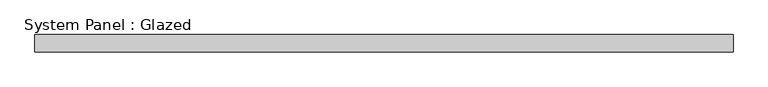
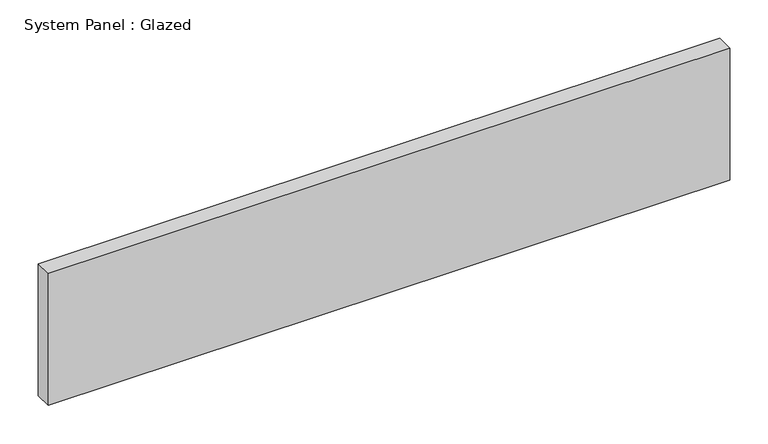
"""IFC4 building model written with IfcOpenShell, lengths in millimetres: plate geometry, System Panel : Glazed."""

from ifc_helpers import new_model, si_unit, origin, origin_with_axes, place, context, project, spatial, polyline, outline, extrude, source, transform, mapped, element, save


def system_panel_glazed_8433226c(model_context):
    return source(origin(), model_context, "Body", "SweptSolid", [
        extrude(outline(polyline([(511.175, 19.05), (-511.175, 19.05), (-511.175, 44.45), (511.175, 44.45), (511.175, 19.05)])), origin_with_axes(), (0.0, 0.0, 1.0), 209.55),
    ])


if __name__ == "__main__":
    model = new_model("IFC4")
    model_context = context("Model", 3, world=origin())
    ifc_project = project(units=[si_unit("LENGTHUNIT", "METRE", prefix="MILLI")], contexts=[model_context])
    site = spatial("IfcSite", under=ifc_project)
    building = spatial("IfcBuilding", under=site)
    placement = place(None, origin())
    system_panel_glazed_shape = system_panel_glazed_8433226c(model_context)
    element("IfcPlate", 1, ObjectType="System Panel : Glazed", at=placement, inside=building, context=model_context, shape_type="MappedRepresentation", body=[
        mapped(system_panel_glazed_shape, transform((0.0, 0.0, 0.0), x_axis=(1.0, 0.0, 0.0), y_axis=(0.0, 1.0, 0.0), z_axis=(0.0, 0.0, 1.0))),
    ])
    save(model, "model.ifc")

# Revit data of these elements
# Type "System Panel : Glazed"
#   Construction Type Id = "GSP4R"
#   Analytic Construction = "1/8 in Pilkington single glazing"
#   Visual Light Transmittance = 0.9
#   Solar Heat Gain Coefficient = 0.86
#   Heat Transfer Coefficient (U) = 1.18115 BTU/(h·ft²·°F)
#   Define Thermal Properties by = 1
# Element 1 (IfcPlate, "System Panel : Glazed")
#   Materials on its faces: "Glass"
# Materials
#   "Glass": class "Glass", colour RGB 0 128 192, transparency 0.75, Description = "Soda Lime Glass", Cost = 0
